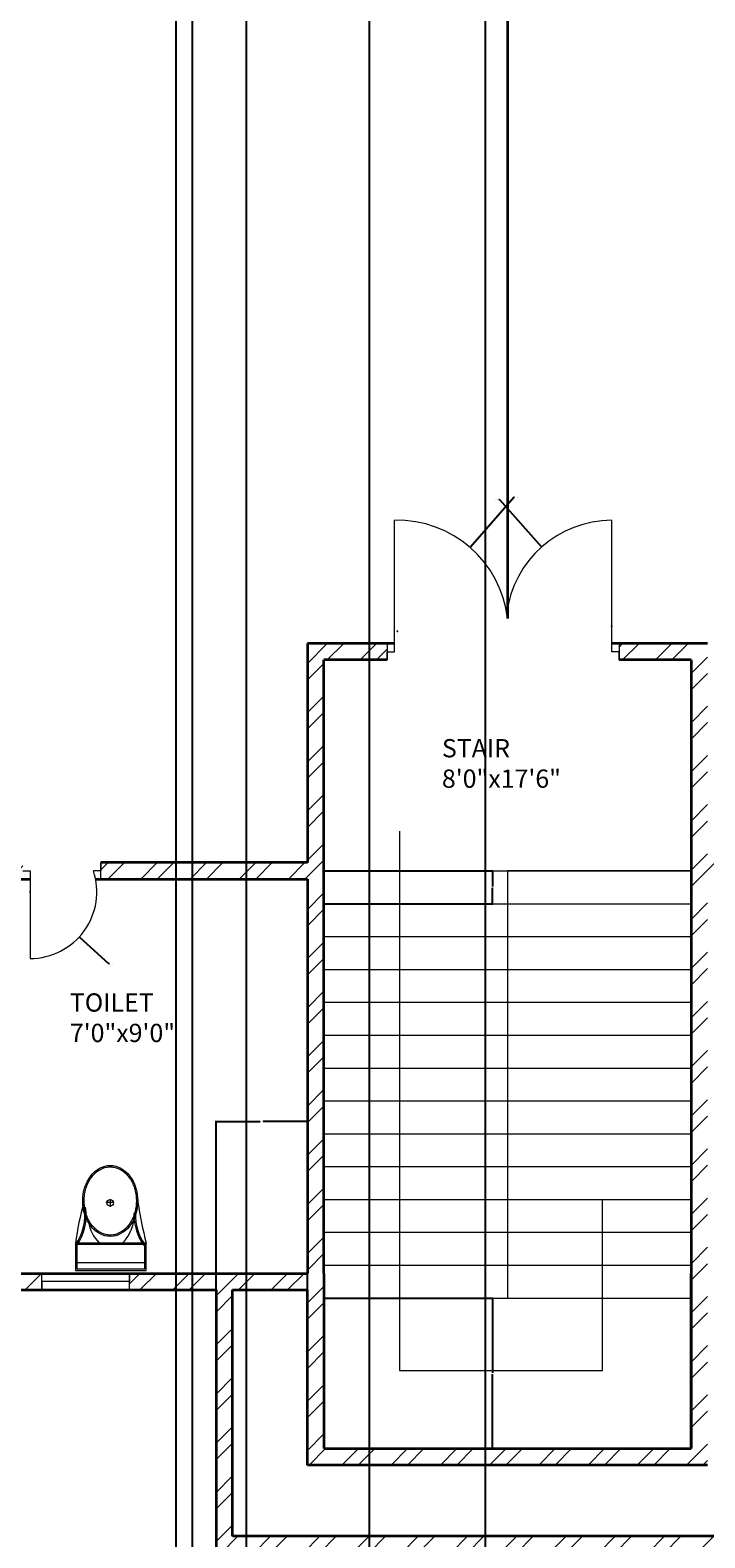
# Model space of a CAD drawing. Units: inches. Extents: x 392 to 1254, y 1207 to 2665.
# Tile 3 of 15: x 702 to 887, y 1414 to 1827. Entities that reach past the tile are written whole.
import ezdxf

# ---------------------------------------------------------------- set-up
doc = ezdxf.new("R2010")
doc.units = ezdxf.units.IN
for name, color, linetype, lineweight in [('A-ANNO-DIMS', 2, 'Continuous', 18), ('A-AREA-IDEN', 7, 'Continuous', 18), ('A-DOOR', 3, 'Continuous', 18), ('A-FLOR-FIXT', 9, 'Continuous', 18), ('A-FLOR-STRS', 7, 'Continuous', 18), ('A-GLAZ', 4, 'Continuous', 18), ('A-WALL', 7, 'Continuous', 35), ('A-WALL-PATT', 252, 'Continuous', 13)]:
    doc.layers.add(name, color=color, linetype=linetype, lineweight=lineweight)
doc.styles.get("Standard").update_dxf_attribs({"font": 'arial.ttf'})
doc.dimstyles.get("Standard").update_dxf_attribs({"dimtxt": 0.18, "dimasz": 0.18, "dimexe": 0.18, "dimexo": 0.0625, "dimgap": 0.09, "dimtad": 0, "dimtih": 1, "dimtoh": 1, "dimdec": 4, "dimzin": 0, "dimdsep": 46, "dimtxsty": 'Standard', "dimcen": 0.09, "dimadec": 0, "dimazin": 0, "dimtfac": 1, "dimtdec": 4, "dimtofl": 0, "dimtmove": 0, "dimatfit": 3, "dimfxl": 1, "dimtolj": 1, "dimtzin": 0, "dimarcsym": 0})

# ---------------------------------------------------------------- blocks, each defined once
blk = doc.blocks.new('A$C31115884')
for p, q in [((283, 498), (223, 498)), ((258, 466), (258, 523)), ((0, 200), (0, 0)), ((520, 200), (0, 200)), ((10, 190), (10, 10)), ((510, 190), (10, 190)), ((510, 10), (510, 190)), ((520, 0), (520, 200)), ((510, 54), (0, 54)), ((10, 10), (510, 10)), ((0, 0), (520, 0))]:
    blk.add_line(p, q)
blk.add_circle((256, 496), 23.6)
for centre, radius, start, end in [((2778, -205), 2807, 165.4549, 171.7133), ((-295, 403), 365, 324.2091, 9.3499), ((-295, 403), 375, 324.2091, 9.3499), ((806, 403), 365, 170.6501, 215.7909), ((3237, 905), 2807, 188.2867, 194.5451), ((384, 406), 293, 190.2774, 224.1564), ((139, 406), 293, 315.8436, 2.6563), ((806, 403), 375, 179.2036, 215.7909)]:
    blk.add_arc(centre, radius, start, end)
blk.add_ellipse((256, 510), major_axis=(0, -261), ratio=0.772727)
blk.add_open_spline([(256, 259), (263, 259), (270, 260), (288, 262), (299, 265), (320, 273), (330, 278), (350, 291), (360, 299), (378, 316), (386, 326), (402, 347), (409, 358), (421, 383), (427, 395), (436, 422), (440, 436), (445, 465), (447, 480), (448, 509), (448, 524), (445, 553), (443, 568), (436, 596), (432, 610), (422, 636), (416, 649), (402, 672), (395, 683), (379, 703), (370, 712), (351, 728), (341, 735), (321, 746), (310, 751), (289, 757), (278, 759), (256, 761), (245, 761), (223, 757), (212, 754), (191, 746), (181, 741), (161, 728), (151, 720), (133, 703), (125, 693), (110, 672), (103, 660), (90, 636), (85, 623), (76, 596), (72, 582), (67, 553), (66, 538), (64, 509), (65, 494), (68, 465), (70, 450), (77, 422), (81, 408), (91, 382), (97, 370), (111, 346), (118, 335), (135, 316), (144, 307), (162, 291), (172, 284), (193, 273), (203, 269), (225, 262), (236, 260), (250, 259), (253, 259), (256, 259)], degree=3, knots=[0, 0, 0, 0, 0.110105, 0.110105, 0.285049, 0.285049, 0.459994, 0.459994, 0.634938, 0.634938, 0.809882, 0.809882, 0.984827, 0.984827, 1.159771, 1.159771, 1.334715, 1.334715, 1.50966, 1.50966, 1.684604, 1.684604, 1.859549, 1.859549, 2.034493, 2.034493, 2.209437, 2.209437, 2.384382, 2.384382, 2.559326, 2.559326, 2.73427, 2.73427, 2.909215, 2.909215, 3.084159, 3.084159, 3.259103, 3.259103, 3.434048, 3.434048, 3.608992, 3.608992, 3.783936, 3.783936, 3.958881, 3.958881, 4.133825, 4.133825, 4.30877, 4.30877, 4.483714, 4.483714, 4.658658, 4.658658, 4.833603, 4.833603, 5.008547, 5.008547, 5.183491, 5.183491, 5.358436, 5.358436, 5.53338, 5.53338, 5.708324, 5.708324, 5.883269, 5.883269, 6.058213, 6.058213, 6.233158, 6.233158, 6.283185, 6.283185, 6.283185, 6.283185])
blk = doc.blocks.new('WIN-24-B')
for p, q in [((2.25, 24), (0, 24)), ((0, 24), (4.5, 24)), ((2.25, 0), (2.25, 24)), ((0, 0), (4.5, 0)), ((4.5, 0), (2.25, 0))]:
    blk.add_line(p, q)
blk = doc.blocks.new('*D25')
at = {"layer": 'A-ANNO-DIMS', "color": 0, "lineweight": -2, "transparency": 16777216}
for p, q in [((541.28, 1482.23), (541.28, 1364.02)), ((1124.78, 1482.23), (1124.78, 1364.02)), ((541.46, 1364.2), (832.64, 1364.2)), ((1124.6, 1364.2), (833.43, 1364.2))]:
    blk.add_line(p, q, dxfattribs=at)
at = {"layer": 'A-ANNO-DIMS', "color": 0, "transparency": 16777216}
for points in [[(541.46, 1364.23), (541.46, 1364.17), (541.28, 1364.2)], [(1124.6, 1364.23), (1124.6, 1364.17), (1124.78, 1364.2)]]:
    blk.add_solid(points, dxfattribs=at)
at = {"layer": 'Defpoints', "color": 0, "transparency": 16777216}
for p in [(541.28, 1482.3), (1124.78, 1482.3), (1124.78, 1364.2)]:
    blk.add_point(p, dxfattribs=at)
at = {"layer": 'A-ANNO-DIMS', "color": 0, "transparency": 16777216, "insert": (833.03, 1364.2), "char_height": 0.18, "attachment_point": 5}
blk.add_mtext('\\A1;583.5', dxfattribs=at)
blk = doc.blocks.new('*D26')
at = {"layer": 'A-ANNO-DIMS', "color": 0, "lineweight": -2, "transparency": 16777216}
for p, q in [((541.22, 2229.3), (495, 2229.3)), ((495.18, 2229.12), (495.18, 1819.98)), ((495.18, 1410.48), (495.18, 1819.61)), ((753.23, 1410.3), (495, 1410.3))]:
    blk.add_line(p, q, dxfattribs=at)
at = {"layer": 'A-ANNO-DIMS', "color": 0, "transparency": 16777216}
for points in [[(495.15, 2229.12), (495.21, 2229.12), (495.18, 2229.3)], [(495.15, 1410.48), (495.21, 1410.48), (495.18, 1410.3)]]:
    blk.add_solid(points, dxfattribs=at)
at = {"layer": 'Defpoints', "color": 0, "transparency": 16777216}
for p in [(495.18, 2229.3), (541.28, 2229.3), (753.29, 1410.3)]:
    blk.add_point(p, dxfattribs=at)
at = {"layer": 'A-ANNO-DIMS', "color": 0, "transparency": 16777216, "insert": (495.18, 1819.8), "char_height": 0.18, "attachment_point": 5}
blk.add_mtext('\\A1;819', dxfattribs=at)
blk = doc.blocks.new('*D29')
at = {"layer": 'A-ANNO-DIMS', "color": 0, "lineweight": -2, "transparency": 16777216}
for p, q in [((541.28, 1482.23), (541.28, 1364.02)), ((753.29, 1410.23), (753.29, 1364.02)), ((541.46, 1364.2), (647, 1364.2)), ((753.11, 1364.2), (647.57, 1364.2))]:
    blk.add_line(p, q, dxfattribs=at)
at = {"layer": 'A-ANNO-DIMS', "color": 0, "transparency": 16777216}
for points in [[(541.46, 1364.23), (541.46, 1364.17), (541.28, 1364.2)], [(753.11, 1364.23), (753.11, 1364.17), (753.29, 1364.2)]]:
    blk.add_solid(points, dxfattribs=at)
at = {"layer": 'Defpoints', "color": 0, "transparency": 16777216}
for p in [(541.28, 1482.3), (753.29, 1410.3), (753.29, 1364.2)]:
    blk.add_point(p, dxfattribs=at)
at = {"layer": 'A-ANNO-DIMS', "color": 0, "transparency": 16777216, "insert": (647.28, 1364.2), "char_height": 0.18, "attachment_point": 5}
blk.add_mtext('\\A1;212', dxfattribs=at)
blk = doc.blocks.new('*D50')
at = {"layer": 'A-ANNO-DIMS', "color": 0, "lineweight": -2, "transparency": 16777216}
for p, q in [((753.29, 1482.36), (753.29, 1528.58)), ((753.47, 1528.4), (765.39, 1528.4)), ((778.1, 1528.4), (766.18, 1528.4)), ((778.28, 1482.36), (778.28, 1528.58))]:
    blk.add_line(p, q, dxfattribs=at)
at = {"layer": 'A-ANNO-DIMS', "color": 0, "transparency": 16777216}
for points in [[(753.47, 1528.43), (753.47, 1528.37), (753.29, 1528.4)], [(778.1, 1528.43), (778.1, 1528.37), (778.28, 1528.4)]]:
    blk.add_solid(points, dxfattribs=at)
at = {"layer": 'Defpoints', "color": 0, "transparency": 16777216}
for p in [(778.28, 1528.4), (753.29, 1482.3), (778.28, 1482.3)]:
    blk.add_point(p, dxfattribs=at)
at = {"layer": 'A-ANNO-DIMS', "color": 0, "transparency": 16777216, "insert": (765.78, 1528.4), "char_height": 0.18, "attachment_point": 5}
blk.add_mtext('\\A1;24.99', dxfattribs=at)
blk = doc.blocks.new('*D52')
at = {"layer": 'A-ANNO-DIMS', "color": 0, "lineweight": -2, "transparency": 16777216}
for p, q in [((782.84, 1480.05), (829.06, 1480.05)), ((828.88, 1479.87), (828.88, 1459.6)), ((828.88, 1438.98), (828.88, 1459.24)), ((782.84, 1438.8), (829.06, 1438.8))]:
    blk.add_line(p, q, dxfattribs=at)
at = {"layer": 'A-ANNO-DIMS', "color": 0, "transparency": 16777216}
for points in [[(828.85, 1479.87), (828.91, 1479.87), (828.88, 1480.05)], [(828.85, 1438.98), (828.91, 1438.98), (828.88, 1438.8)]]:
    blk.add_solid(points, dxfattribs=at)
at = {"layer": 'Defpoints', "color": 0, "transparency": 16777216}
for p in [(782.78, 1480.05), (782.78, 1438.8), (828.88, 1438.8)]:
    blk.add_point(p, dxfattribs=at)
at = {"layer": 'A-ANNO-DIMS', "color": 0, "transparency": 16777216, "insert": (828.88, 1459.42), "char_height": 0.18, "attachment_point": 5}
blk.add_mtext('\\A1;41.25', dxfattribs=at)
blk = doc.blocks.new('*D53')
at = {"layer": 'A-ANNO-DIMS', "color": 0, "lineweight": -2, "transparency": 16777216}
for p, q in [((782.84, 1597.05), (829.06, 1597.05)), ((828.88, 1596.87), (828.88, 1592.73)), ((828.88, 1588.23), (828.88, 1592.36)), ((782.84, 1588.05), (829.06, 1588.05))]:
    blk.add_line(p, q, dxfattribs=at)
at = {"layer": 'A-ANNO-DIMS', "color": 0, "transparency": 16777216}
for points in [[(828.85, 1596.87), (828.91, 1596.87), (828.88, 1597.05)], [(828.85, 1588.23), (828.91, 1588.23), (828.88, 1588.05)]]:
    blk.add_solid(points, dxfattribs=at)
at = {"layer": 'Defpoints', "color": 0, "transparency": 16777216}
for p in [(782.78, 1597.05), (782.78, 1588.05), (828.88, 1588.05)]:
    blk.add_point(p, dxfattribs=at)
at = {"layer": 'A-ANNO-DIMS', "color": 0, "transparency": 16777216, "insert": (828.88, 1592.55), "char_height": 0.18, "attachment_point": 5}
blk.add_mtext('\\A1;9', dxfattribs=at)
blk = doc.blocks.new('*D75')
at = {"layer": 'A-ANNO-DIMS', "color": 0, "lineweight": -2, "transparency": 16777216}
for p, q in [((746.78, 2056.73), (746.78, 1364.02)), ((742.28, 2052.23), (742.28, 1364.02)), ((742.46, 1364.2), (744.27, 1364.2)), ((746.6, 1364.2), (744.79, 1364.2))]:
    blk.add_line(p, q, dxfattribs=at)
at = {"layer": 'A-ANNO-DIMS', "color": 0, "transparency": 16777216}
for points in [[(742.46, 1364.23), (742.46, 1364.17), (742.28, 1364.2)], [(746.6, 1364.23), (746.6, 1364.17), (746.78, 1364.2)]]:
    blk.add_solid(points, dxfattribs=at)
at = {"layer": 'Defpoints', "color": 0, "transparency": 16777216}
for p in [(746.78, 2056.8), (742.28, 2052.3), (746.78, 1364.2)]:
    blk.add_point(p, dxfattribs=at)
at = {"layer": 'A-ANNO-DIMS', "color": 0, "transparency": 16777216, "insert": (744.53, 1364.2), "char_height": 0.18, "attachment_point": 5}
blk.add_mtext('\\A1;4.5', dxfattribs=at)
blk = doc.blocks.new('*D78')
at = {"layer": 'A-ANNO-DIMS', "color": 0, "lineweight": -2, "transparency": 16777216}
for p, q in [((746.78, 2056.73), (746.78, 1364.02)), ((761.56, 2056.73), (761.56, 1364.02)), ((746.96, 1364.2), (753.72, 1364.2)), ((761.38, 1364.2), (754.63, 1364.2))]:
    blk.add_line(p, q, dxfattribs=at)
at = {"layer": 'A-ANNO-DIMS', "color": 0, "transparency": 16777216}
for points in [[(746.96, 1364.23), (746.96, 1364.17), (746.78, 1364.2)], [(761.38, 1364.23), (761.38, 1364.17), (761.56, 1364.2)]]:
    blk.add_solid(points, dxfattribs=at)
at = {"layer": 'Defpoints', "color": 0, "transparency": 16777216}
for p in [(746.78, 2056.8), (761.56, 2056.8), (761.56, 1364.2)]:
    blk.add_point(p, dxfattribs=at)
at = {"layer": 'A-ANNO-DIMS', "color": 0, "transparency": 16777216, "insert": (754.17, 1364.2), "char_height": 0.18, "attachment_point": 5}
blk.add_mtext('\\A1;14.782', dxfattribs=at)
blk = doc.blocks.new('*D80')
at = {"layer": 'A-ANNO-DIMS', "color": 0, "lineweight": -2, "transparency": 16777216}
for p, q in [((795.21, 2052.23), (795.21, 1364.02)), ((826.91, 2052.23), (826.91, 1364.02)), ((795.39, 1364.2), (810.6, 1364.2)), ((826.73, 1364.2), (811.52, 1364.2))]:
    blk.add_line(p, q, dxfattribs=at)
at = {"layer": 'A-ANNO-DIMS', "color": 0, "transparency": 16777216}
for points in [[(795.39, 1364.23), (795.39, 1364.17), (795.21, 1364.2)], [(826.73, 1364.23), (826.73, 1364.17), (826.91, 1364.2)]]:
    blk.add_solid(points, dxfattribs=at)
at = {"layer": 'Defpoints', "color": 0, "transparency": 16777216}
for p in [(795.21, 2052.3), (826.91, 2052.3), (826.91, 1364.2)]:
    blk.add_point(p, dxfattribs=at)
at = {"layer": 'A-ANNO-DIMS', "color": 0, "transparency": 16777216, "insert": (811.06, 1364.2), "char_height": 0.18, "attachment_point": 5}
blk.add_mtext('\\A1;31.694', dxfattribs=at)
blk = doc.blocks.new('*D85')
at = {"layer": 'A-ANNO-DIMS', "color": 0, "lineweight": -2, "transparency": 16777216}
for p, q in [((834.75, 1699.34), (822.93, 1685.74)), ((834.93, 1699.34), (834.75, 1699.34)), ((802.81, 1662.73), (802.99, 1662.73)), ((802.9, 1662.64), (802.9, 1662.82))]:
    blk.add_line(p, q, dxfattribs=at)
at = {"layer": 'A-ANNO-DIMS', "color": 0, "transparency": 16777216}
blk.add_solid([(822.9, 1685.76), (822.95, 1685.72), (822.81, 1685.61)], dxfattribs=at)
at = {"layer": 'Defpoints', "color": 0, "transparency": 16777216}
for p in [(822.81, 1685.61), (802.9, 1662.73)]:
    blk.add_point(p, dxfattribs=at)
at = {"layer": 'A-ANNO-DIMS', "color": 0, "transparency": 16777216, "insert": (835.41, 1699.34), "char_height": 0.18, "attachment_point": 5}
blk.add_mtext('\\A1;R30.33', dxfattribs=at)
blk = doc.blocks.new('*D86')
at = {"layer": 'A-ANNO-DIMS', "color": 0, "lineweight": -2, "transparency": 16777216}
for p, q in [((830.67, 1698.75), (830.85, 1698.75)), ((830.85, 1698.75), (842.26, 1685.89)), ((861.59, 1664), (861.59, 1664.18)), ((861.5, 1664.09), (861.68, 1664.09))]:
    blk.add_line(p, q, dxfattribs=at)
at = {"layer": 'A-ANNO-DIMS', "color": 0, "transparency": 16777216}
blk.add_solid([(842.28, 1685.91), (842.24, 1685.87), (842.38, 1685.75)], dxfattribs=at)
at = {"layer": 'Defpoints', "color": 0, "transparency": 16777216}
for p in [(842.38, 1685.75), (861.59, 1664.09)]:
    blk.add_point(p, dxfattribs=at)
at = {"layer": 'A-ANNO-DIMS', "color": 0, "transparency": 16777216, "insert": (830.12, 1698.75), "char_height": 0.18, "attachment_point": 5}
blk.add_mtext('\\A1;R28.956', dxfattribs=at)
blk = doc.blocks.new('*D103')
at = {"layer": 'A-ANNO-DIMS', "color": 0, "lineweight": -2, "transparency": 16777216}
for p, q in [((702.33, 1591.29), (702.51, 1591.29)), ((702.42, 1591.2), (702.42, 1591.38)), ((723.92, 1571.54), (715.99, 1578.83)), ((724.1, 1571.54), (723.92, 1571.54))]:
    blk.add_line(p, q, dxfattribs=at)
at = {"layer": 'A-ANNO-DIMS', "color": 0, "transparency": 16777216}
blk.add_solid([(716.01, 1578.85), (715.97, 1578.81), (715.86, 1578.95)], dxfattribs=at)
at = {"layer": 'Defpoints', "color": 0, "transparency": 16777216}
for p in [(702.42, 1591.29), (715.86, 1578.95)]:
    blk.add_point(p, dxfattribs=at)
at = {"layer": 'A-ANNO-DIMS', "color": 0, "transparency": 16777216, "insert": (724.65, 1571.54), "char_height": 0.18, "attachment_point": 5}
blk.add_mtext('\\A1;R18.247', dxfattribs=at)

msp = doc.modelspace()

# ---------------------------------------------------------------- hatches: boundary and pattern name
at = {"layer": 'A-WALL-PATT'}
h = msp.add_hatch(dxfattribs=at)
h.set_pattern_fill('ANSI32', color=256)
h.paths.add_polyline_path([(579.5309, 2227.0453), (579.5309, 2229.2953), (541.2807, 2229.2953), (541.2807, 2182.3091), (545.7807, 2182.3091), (545.7807, 2224.7953), (579.5309, 2224.7953)])
h.paths.add_polyline_path([(655.4442, 2229.2953), (627.5309, 2229.2953), (627.5309, 2224.7953), (655.4442, 2224.7953), (655.4442, 2227.0453)])
h.paths.add_polyline_path([(703.0758, 2229.2953), (678.5257, 2229.2953), (678.5257, 2227.0453), (678.5257, 2224.7953), (689.7807, 2224.7953), (689.7807, 2158.6973), (694.2807, 2158.6973), (694.2807, 2224.7953), (703.0758, 2224.7953)])
h.paths.add_polyline_path([(768.5767, 2229.2953), (727.0758, 2229.2953), (727.0758, 2224.7953), (742.2807, 2224.7953), (742.2807, 2128.7953), (694.2807, 2128.7953), (694.2807, 2134.0554), (689.7807, 2134.0554), (689.7807, 2090.2854), (694.2807, 2090.2854), (694.2807, 2124.2953), (742.2807, 2124.2953), (742.2807, 2052.2953), (795.2123, 2052.2953), (795.2123, 2054.5453), (795.2123, 2056.7953), (746.7807, 2056.7953), (746.7807, 2224.7953), (768.5767, 2224.7953)])
h.paths.add_polyline_path([(867.5089, 2229.2953), (804.5767, 2229.2953), (804.5767, 2224.7953), (830.7807, 2224.7953), (830.7807, 2056.7953), (826.9066, 2056.7953), (826.9066, 2052.2953), (830.7807, 2052.2953), (830.7807, 1886.6777, -0.01766664), (830.8602, 1884.2953), (835.0818, 1884.2953, -0.04411348), (835.2807, 1889.9369), (835.2807, 2052.2953), (839.418, 2052.2953), (839.418, 2056.7953), (835.2807, 2056.7953), (835.2807, 2224.7953), (867.5089, 2224.7953)])
h.paths.add_polyline_path([(939.8604, 2229.2953), (903.5089, 2229.2953), (903.5089, 2227.0453), (903.5089, 2224.7953), (919.2807, 2224.7953), (919.2807, 2056.7953), (870.6499, 2056.7953), (870.6499, 2052.2953), (923.7807, 2052.2953), (923.7807, 2124.2953), (971.7807, 2124.2953), (971.7807, 2089.7112), (974.0307, 2089.7112), (976.2807, 2089.7112), (976.2807, 2133.56), (974.0307, 2133.56), (971.7807, 2133.56), (971.7807, 2128.7953), (923.7807, 2128.7953), (923.7807, 2224.7953), (939.8604, 2224.7953)])
h.paths.add_polyline_path([(1124.7807, 2229.2953), (1009.403, 2229.2953), (1009.403, 2224.7953), (1120.2807, 2224.7953), (1120.2807, 2184.7605), (1124.7807, 2184.7605)])
h.paths.add_polyline_path([(1124.7807, 2124.7605), (1120.2807, 2124.7605), (1120.2807, 2056.7953), (976.2807, 2056.7953), (976.2807, 2061.471), (971.7807, 2061.471), (971.7807, 2047.7483), (974.0307, 2047.7483), (976.2807, 2047.7483), (976.2807, 2052.2953), (1120.2807, 2052.2953), (1120.2807, 1992.457), (1124.7807, 1992.457)])
h.paths.add_polyline_path([(1124.7807, 1932.457), (1122.5307, 1932.457), (1120.2807, 1932.457), (1120.2807, 1884.2953), (976.2807, 1884.2953), (976.2807, 2019.9536), (971.7807, 2019.9536), (971.7807, 1884.2953), (869.0911, 1884.2953), (869.0911, 1879.7953), (971.7807, 1879.7953), (1013.7807, 1879.7953), (1013.7807, 1831.7953), (971.7807, 1831.7953), (971.7807, 1822.3831), (974.0307, 1822.3831), (976.2807, 1822.3831), (976.2807, 1827.2953), (1013.7807, 1827.2953), (1025.6191, 1827.2953), (1025.6191, 1829.5453), (1025.6191, 1831.7953), (1018.2807, 1831.7953), (1018.2807, 1879.7953), (1120.2807, 1879.7953), (1120.2807, 1866.9192), (1124.7807, 1866.9192)])
h.paths.add_polyline_path([(1124.7807, 1842.9192), (1122.5307, 1842.9192), (1120.2807, 1842.9192), (1120.2807, 1831.7953), (1050.2021, 1831.7953), (1050.2021, 1827.2953), (1120.2807, 1827.2953), (1120.2807, 1781.4559), (1124.7807, 1781.4559)])
h.paths.add_polyline_path([(976.2807, 1790.8718), (971.7807, 1790.8718), (971.7807, 1648.3339), (976.2807, 1648.3339), (976.2807, 1654.7953), (1120.2807, 1654.7953), (1120.2807, 1626.3807), (1124.7807, 1626.3807), (1124.7807, 1721.4559), (1120.2807, 1721.4559), (1120.2807, 1659.2953), (976.2807, 1659.2953)])
h.paths.add_polyline_path([(1124.7807, 1566.3807), (1120.2807, 1566.3807), (1120.2807, 1486.7953), (1101.07, 1486.7953), (1101.07, 1482.2953), (1124.7807, 1482.2953)])
h.paths.add_polyline_path([(1041.07, 1484.5453), (1041.07, 1486.7953), (1006.2807, 1486.7953), (1006.2807, 1484.5453), (1006.2807, 1482.2953), (1041.07, 1482.2953)])
h.paths.add_polyline_path([(976.2807, 1617.5497), (974.0307, 1617.5497), (971.7807, 1617.5497), (971.7807, 1599.2953), (965.8041, 1599.2953), (965.8041, 1594.7953), (971.7807, 1594.7953), (971.7807, 1486.7953), (954.1249, 1486.7953), (954.1249, 1482.2953), (981.5717, 1482.2953), (981.5717, 1484.5453), (981.5717, 1486.7953), (976.2807, 1486.7953)])
h.paths.add_polyline_path([(930.1249, 1486.7953), (887.7807, 1486.7953), (887.7807, 1594.7953), (941.9141, 1594.7953), (941.9141, 1597.0453), (941.9141, 1599.2953), (887.7807, 1599.2953), (887.7807, 1659.2953), (863.5916, 1659.2953), (863.5916, 1654.7953), (883.2807, 1654.7953), (883.2807, 1438.7953), (782.7807, 1438.7953), (782.7807, 1486.7953), (782.7807, 1654.7953), (800.1309, 1654.7953), (800.1309, 1657.0453), (800.1309, 1659.2953), (778.2807, 1659.2953), (778.2807, 1599.2953), (721.7333, 1599.2953), (721.7333, 1597.0453), (721.7333, 1594.7953), (778.2807, 1594.7953), (778.2807, 1486.7953), (729.598, 1486.7953), (729.598, 1482.2953), (753.2885, 1482.2953), (753.2885, 1410.2953), (922.9852, 1410.2953), (922.9852, 1482.2953), (930.1249, 1482.2953)])
h.paths.add_polyline_path([(918.4852, 1482.2953), (918.4852, 1414.7953), (757.7885, 1414.7953), (757.7885, 1482.2953), (778.2807, 1482.2953), (778.2807, 1434.2953), (782.7807, 1434.2953), (887.7807, 1434.2953), (887.7807, 1438.7953), (887.7807, 1482.2953)], flags=16)
h.paths.add_polyline_path([(694.2807, 1594.7953), (700.4169, 1594.7953), (700.4169, 1597.0453), (700.4169, 1599.2953), (694.2807, 1599.2953), (694.2807, 1617.7503), (692.0307, 1617.7503), (689.7807, 1617.7503), (689.7807, 1486.7953), (682.7672, 1486.7953), (682.7672, 1482.2953), (705.598, 1482.2953), (705.598, 1484.5453), (705.598, 1486.7953), (694.2807, 1486.7953)])
h.paths.add_polyline_path([(545.7807, 1654.7953), (689.7807, 1654.7953), (689.7807, 1649.7691), (694.2807, 1649.7691), (694.2807, 1789.3981), (692.0307, 1789.3981), (689.7807, 1789.3981), (689.7807, 1659.2953), (545.7807, 1659.2953), (545.7807, 1714.4681), (543.5307, 1714.4681), (541.2807, 1714.4681), (541.2807, 1482.2953), (567.0628, 1482.2953), (567.0628, 1484.5453), (567.0628, 1486.7953), (545.7807, 1486.7953)])
h.paths.add_polyline_path([(545.7807, 1827.2953), (620.2247, 1827.2953), (620.2247, 1829.5453), (620.2247, 1831.7953), (545.7807, 1831.7953), (545.7807, 1846.8518), (541.2807, 1846.8518), (541.2807, 1774.4681), (545.7807, 1774.4681)])
h.paths.add_polyline_path([(797.0944, 1884.2953), (694.2807, 1884.2953), (694.2807, 2019.0288), (692.0307, 2019.0288), (689.7807, 2019.0288), (689.7807, 1884.2953), (545.7807, 1884.2953), (545.7807, 1951.8244), (541.2807, 1951.8244), (541.2807, 1870.8518), (543.5307, 1870.8518), (545.7807, 1870.8518), (545.7807, 1879.7953), (647.7807, 1879.7953), (647.7807, 1831.7953), (642.6413, 1831.7953), (642.6413, 1827.2953), (652.2807, 1827.2953), (689.7807, 1827.2953), (689.7807, 1821.0531), (694.2807, 1821.0531), (694.2807, 1831.7953), (652.2807, 1831.7953), (652.2807, 1879.7953), (797.0944, 1879.7953), (797.0944, 1882.0453)])
h.paths.add_polyline_path([(545.7807, 2122.3091), (541.2807, 2122.3091), (541.2807, 2011.8244), (543.5307, 2011.8244), (545.7807, 2011.8244), (545.7807, 2052.2953), (689.7807, 2052.2953), (689.7807, 2048.2048), (694.2807, 2048.2048), (694.2807, 2061.3129), (692.0307, 2061.3129), (689.7807, 2061.3129), (689.7807, 2056.7953), (545.7807, 2056.7953)])

# ---------------------------------------------------------------- linework, layer by layer
at = {"layer": 'A-DOOR'}
for p, q in [((802.1309, 1657.0453), (802.1309, 1693.0453)), ((861.5916, 1657.0453), (861.5916, 1693.0453)), ((800.1309, 1659.2953), (800.1309, 1654.7953)), ((800.1309, 1654.7953), (800.1309, 1657.0453)), ((800.1309, 1657.0453), (802.1309, 1657.0453)), ((863.5916, 1657.0453), (861.5916, 1657.0453)), ((863.5916, 1659.2953), (863.5916, 1654.7953)), ((863.5916, 1654.7953), (863.5916, 1657.0453)), ((721.7333, 1594.7953), (721.7333, 1599.2953)), ((721.7333, 1599.2953), (721.7333, 1597.0453)), ((700.4169, 1597.0453), (702.4169, 1597.0453)), ((702.4169, 1597.0453), (702.4169, 1573.0453)), ((721.7333, 1597.0453), (719.7333, 1597.0453))]:
    msp.add_line(p, q, dxfattribs=at)
for centre, radius, start, end in [((802.9006, 1662.7258), 30.3293, 6.494553, 91.454172), ((861.5916, 1664.0893), 28.956, 90, 173.131827), ((702.4169, 1591.2923), 18.247, 270, 18.37786)]:
    msp.add_arc(centre, radius, start, end, dxfattribs=at)
at = {"layer": 'A-FLOR-STRS'}
for p, q in [((803.4518, 1607.9183), (803.4518, 1460.1588)), ((782.7807, 1597.0453), (883.2807, 1597.0453)), ((883.2807, 1597.0453), (833.0307, 1597.0453)), ((833.0307, 1597.0453), (833.0307, 1480.0453)), ((782.7807, 1588.0453), (883.2807, 1588.0453)), ((782.7807, 1579.0453), (883.2807, 1579.0453)), ((782.7807, 1570.0453), (883.2807, 1570.0453)), ((782.7807, 1561.0453), (883.2807, 1561.0453)), ((782.7807, 1552.0453), (883.2807, 1552.0453)), ((782.7807, 1543.0453), (883.2807, 1543.0453)), ((782.7807, 1534.0453), (883.2807, 1534.0453)), ((782.7807, 1525.0453), (883.2807, 1525.0453)), ((782.7807, 1516.0453), (883.2807, 1516.0453)), ((782.7807, 1507.0453), (883.2807, 1507.0453)), ((859.0064, 1460.1588), (859.0064, 1507.0453)), ((782.7807, 1498.0453), (883.2807, 1498.0453)), ((782.7807, 1489.0453), (883.2807, 1489.0453)), ((782.7807, 1480.0453), (883.2807, 1480.0453)), ((803.4518, 1460.1588), (859.0064, 1460.1588))]:
    msp.add_line(p, q, dxfattribs=at)
at = {"layer": 'A-WALL'}
for p, q in [((833.0352, 1879.7953), (833.0352, 1674.6213)), ((833.0352, 1674.6213), (833.0352, 1666.1563)), ((778.2807, 1659.2953), (778.2807, 1599.2953)), ((802.1309, 1659.2953), (778.2807, 1659.2953)), ((887.7807, 1659.2953), (861.5916, 1659.2953)), ((782.7807, 1486.7953), (782.7807, 1654.7953)), ((800.1309, 1654.7953), (782.7807, 1654.7953)), ((883.2807, 1654.7953), (863.5916, 1654.7953)), ((883.2807, 1654.7953), (883.2807, 1438.7953)), ((778.2807, 1599.2953), (721.7333, 1599.2953)), ((782.7807, 1594.7953), (782.7807, 1599.2953)), ((694.2807, 1594.7953), (702.4169, 1594.7953)), ((720.3246, 1594.7953), (778.2807, 1594.7953)), ((778.2807, 1594.7953), (778.2807, 1486.7953)), ((694.2807, 1486.7953), (778.2807, 1486.7953)), ((782.7807, 1486.7953), (782.7807, 1438.7953)), ((883.2807, 1438.7953), (883.2807, 1486.7953)), ((680.7672, 1482.2953), (753.2885, 1482.2953)), ((753.2885, 1482.2953), (753.2885, 1410.2953)), ((757.7885, 1414.7953), (757.7885, 1482.2953)), ((757.7885, 1482.2953), (778.2807, 1482.2953)), ((778.2807, 1434.2953), (778.2807, 1482.2953)), ((782.7807, 1438.7953), (883.2807, 1438.7953)), ((782.7807, 1434.2953), (778.2807, 1434.2953)), ((887.7807, 1434.2953), (782.7807, 1434.2953)), ((918.4852, 1414.7953), (757.7885, 1414.7953))]:
    msp.add_line(p, q, dxfattribs=at)

# ---------------------------------------------------------------- block references
at = {"layer": 'A-FLOR-FIXT', "xscale": 0.0372717239612423, "yscale": 0.0372717239612423, "zscale": 0.0372717239612423}
msp.add_blockref('A$C31115884', (714.7813, 1487.6334), dxfattribs=at)
at = {"layer": 'A-GLAZ', "rotation": 90}
msp.add_blockref('WIN-24-B', (729.5982, 1482.2956), dxfattribs=at)

# ---------------------------------------------------------------- texts
at = {"layer": 'A-AREA-IDEN', "char_height": 5, "attachment_point": 1}
for s, width, insert in [('STAIR\\P8\'0"x17\'6"', 124.534325, (815.0815, 1633.1333)), ('TOILET\\P7\'0"x9\'0"', 107.19739, (713.2717, 1563.487))]:
    msp.add_mtext_dynamic_manual_height_columns(s, width=width, gutter_width=12.5, heights=[0], dxfattribs=dict(at, insert=insert))

# ---------------------------------------------------------------- dimensions: what is measured, and where the dimension line sits
at = {"layer": 'A-ANNO-DIMS'}
for base, p1, p2, angle, override, picture, middle in [((495.1807, 2229.2953), (753.2885, 1410.2953), (541.2807, 2229.2953), 90, {"dimdec": 0, "dimlfac": 1, "dimrnd": 0, "dimzin": 0, "dimdsep": 46, "dimlunit": 2}, '*D26', (495.1807, 1819.7953)), ((828.8807, 1588.0453), (782.7807, 1597.0453), (782.7807, 1588.0453), 270, {"dimdec": 0, "dimlfac": 1, "dimrnd": 0, "dimzin": 0, "dimdsep": 46, "dimlunit": 2}, '*D53', (828.8807, 1592.5453)), ((828.8807, 1438.7953), (782.7807, 1480.0453), (782.7807, 1438.7953), 270, {"dimdec": 2, "dimlfac": 1, "dimrnd": 0, "dimzin": 0, "dimdsep": 46, "dimlunit": 2}, '*D52', (828.8807, 1459.4203))]:
    dim = msp.add_linear_dim(base=base, p1=p1, p2=p2, angle=angle, dimstyle='Standard', override=override, dxfattribs=at)
    dim.commit()
    dim.dimension.update_dxf_attribs({"geometry": picture, "text_midpoint": middle})
for base, p1, p2, override, picture, middle in [((746.7807, 1364.1953), (742.2807, 2052.2953), (746.7807, 2056.7953), {"dimdec": 1, "dimlfac": 1, "dimrnd": 0, "dimzin": 0, "dimdsep": 46, "dimlunit": 2}, '*D75', (744.5307, 1364.1953)), ((761.5625, 1364.1953), (746.7807, 2056.7953), (761.5625, 2056.7953), {"dimdec": 3, "dimlfac": 1, "dimrnd": 0, "dimzin": 0, "dimdsep": 46, "dimlunit": 2}, '*D78', (754.1716, 1364.1953)), ((826.9066, 1364.1953), (795.2123, 2052.2953), (826.9066, 2052.2953), {"dimdec": 3, "dimlfac": 1, "dimrnd": 0, "dimzin": 0, "dimdsep": 46, "dimlunit": 2}, '*D80', (811.0595, 1364.1953)), ((778.2807, 1528.3953), (753.2885, 1482.2953), (778.2807, 1482.2953), {"dimdec": 2, "dimlfac": 1, "dimrnd": 0, "dimzin": 0, "dimdsep": 46, "dimlunit": 2}, '*D50', (765.7846, 1528.3953)), ((1124.7807, 1364.1953), (541.2807, 1482.2953), (1124.7807, 1482.2953), {"dimdec": 1, "dimlfac": 1, "dimrnd": 0, "dimzin": 0, "dimdsep": 46, "dimlunit": 2}, '*D25', (833.0307, 1364.1953)), ((753.2885, 1364.1953), (541.2807, 1482.2953), (753.2885, 1410.2953), {"dimdec": 0, "dimlfac": 1, "dimrnd": 0, "dimzin": 0, "dimdsep": 46, "dimlunit": 2}, '*D29', (647.2846, 1364.1953))]:
    dim = msp.add_linear_dim(base=base, p1=p1, p2=p2, dimstyle='Standard', override=override, dxfattribs=at)
    dim.commit()
    dim.dimension.update_dxf_attribs({"geometry": picture, "text_midpoint": middle})
for center, mpoint, override, picture, middle in [((802.9006, 1662.7258), (822.8087, 1685.6066), {"dimdec": 2, "dimlfac": 1, "dimrnd": 0, "dimzin": 0, "dimdsep": 46, "dimlunit": 2}, '*D85', (835.4134, 1699.3351)), ((861.5916, 1664.0893), (842.3799, 1685.7541), {"dimdec": 3, "dimlfac": 1, "dimrnd": 0, "dimzin": 0, "dimdsep": 46, "dimlunit": 2}, '*D86', (830.1232, 1698.753)), ((702.4169, 1591.2923), (715.8555, 1578.949), {"dimdec": 3, "dimlfac": 1, "dimrnd": 0, "dimzin": 0, "dimdsep": 46, "dimlunit": 2}, '*D103', (724.6484, 1571.543))]:
    dim = msp.add_radius_dim(center=center, mpoint=mpoint, dimstyle='Standard', override=override, dxfattribs=at)
    dim.commit()
    dim.dimension.update_dxf_attribs({"geometry": picture, "text_midpoint": middle, "dimtype": 164})

doc.saveas('drawing.dxf')
